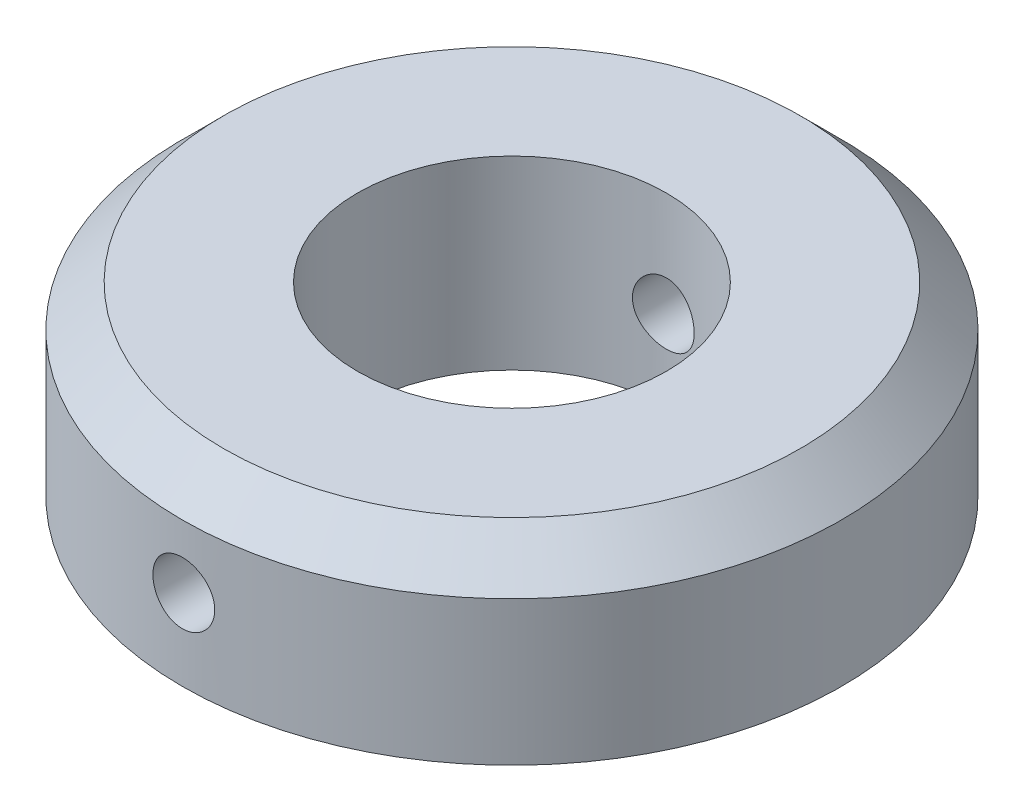
SolidWorks part; units mm, degrees
material "Plain Carbon Steel"
ref_plane "Front Plane" through (0, 0, 0) normal (0, 0, 1) x (1, 0, 0)
ref_plane "Top Plane" through (0, 0, 0) normal (0, 1, 0) x (1, 0, 0)
ref_plane "Right Plane" through (0, 0, 0) normal (1, 0, 0) x (0, 0, -1)
sketch "Collar Ring Profile" plane through (0, 0, 0) normal (0, 1, 0) x (1, 0, 0)
  circle A0 centre (0, 0) radius 16
  circle A1 centre (0, 0) radius 7.5
  dimension "D1" = 32
  dimension "D2" = 15
extrude "Collar Body" add sketch "Collar Ring Profile" along normal blind 9
chamfer "Edge Chamfer 2x45" distance 2 angle 45 1 edges at (0, 9, 16)
sketch "Cross Hole Profile" plane through (0, 0, 0) normal (0, 0, 1) x (1, 0, 0)
  circle A0 centre (0, 3.9303) radius 1.5
  dimension "D1" = 3
  dimension "D2" = 3.9303
extrude "Cross Hole Ø3" cut sketch "Cross Hole Profile" against normal through all both and the other way through all
